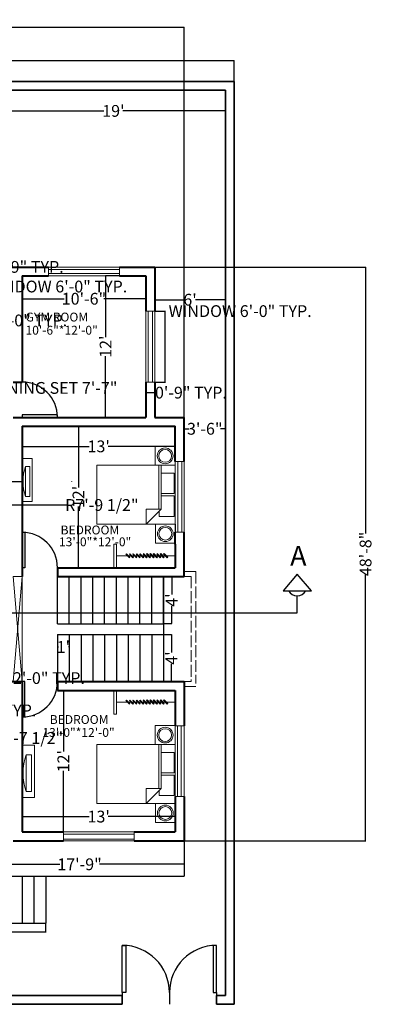
# Model space of a CAD drawing. Units: inches. Extents: x 1146 to 2917, y 889 to 2437.
# Tile 9 of 13: x 1792 to 2152, y 1432 to 2434. Entities that reach past the tile are written whole.
import ezdxf

# ---------------------------------------------------------------- set-up
doc = ezdxf.new("R2010")
doc.units = ezdxf.units.IN
doc.header["$MEASUREMENT"] = 0
doc.linetypes.add('ACAD_ISO02W100', pattern=[15, 12, -3])
for name, color, linetype, lineweight in [('A-ANNO-DIMS', 2, 'Continuous', 18), ('A-ANNO-SYMB', 7, 'Continuous', 25), ('A-AREA-IDEN', 7, 'Continuous', 18), ('A-FLOR-CASE', 9, 'Continuous', 20), ('A-FURN', 9, 'Continuous', 18), ('A-SITE-GATE', 10, 'Continuous', 25), ('A-SITE-WALL', 7, 'Continuous', 35), ('curtain wall', 70, 'ACAD_ISO02W100', 18), ('door', 10, 'Continuous', 25), ('openings', 130, 'Continuous', 18), ('staircase', 6, 'Continuous', 25), ('wall', 7, 'Continuous', 40), ('window', 5, 'Continuous', 18)]:
    doc.layers.add(name, color=color, linetype=linetype, lineweight=lineweight)
doc.styles.get("Standard").update_dxf_attribs({"font": 'arial.ttf'})
doc.dimstyles.new('Copy of Standard', dxfattribs={"dimtxt": 24, "dimasz": 0.18, "dimexe": 0.18, "dimexo": 0.0625, "dimgap": 0.09, "dimtad": 0, "dimtoh": 1, "dimdec": 1, "dimzin": 0, "dimdsep": 46, "dimlunit": 4, "dimtxsty": 'Standard', "dimcen": 0.09, "dimadec": 0, "dimazin": 0, "dimtfac": 1, "dimtdec": 1, "dimtofl": 0, "dimtmove": 0, "dimatfit": 3, "dimfxl": 1, "dimtolj": 1, "dimtzin": 0, "dimarcsym": 0})
doc.dimstyles.get("Standard").update_dxf_attribs({"dimtxt": 12, "dimasz": 0.18, "dimexe": 0.18, "dimexo": 0.0625, "dimgap": 0.09, "dimtad": 0, "dimtoh": 1, "dimdec": 1, "dimzin": 0, "dimdsep": 46, "dimlunit": 4, "dimtxsty": 'Standard', "dimcen": 0.09, "dimadec": 0, "dimazin": 0, "dimtfac": 1, "dimtdec": 1, "dimtofl": 0, "dimtmove": 0, "dimatfit": 3, "dimfxl": 1, "dimtolj": 1, "dimtzin": 0, "dimarcsym": 0})

# ---------------------------------------------------------------- blocks, each defined once
blk = doc.blocks.new('*D7')
at = {"layer": 'A-ANNO-DIMS', "color": 0, "lineweight": -2, "transparency": 16777216}
for p, q in [((1929.1, 2182.3), (1929.1, 2149)), ((2001.1, 2182.3), (2001.1, 2149)), ((1929.3, 2149.2), (1959.5, 2149.2)), ((2001, 2149.2), (1970.8, 2149.2))]:
    blk.add_line(p, q, dxfattribs=at)
at = {"layer": 'A-ANNO-DIMS', "color": 0, "transparency": 16777216}
for points in [[(1929.3, 2149.2), (1929.3, 2149.1), (1929.1, 2149.2)], [(2001, 2149.2), (2001, 2149.1), (2001.1, 2149.2)]]:
    blk.add_solid(points, dxfattribs=at)
at = {"layer": 'Defpoints', "color": 0, "transparency": 16777216}
for p in [(1929.1, 2182.4), (2001.1, 2182.4), (2001.1, 2149.2)]:
    blk.add_point(p, dxfattribs=at)
at = {"layer": 'A-ANNO-DIMS', "color": 0, "transparency": 16777216, "insert": (1965.1, 2149.2), "char_height": 12, "attachment_point": 5}
blk.add_mtext("\\A1;6'", dxfattribs=at)
blk = doc.blocks.new('*D8')
at = {"layer": 'A-ANNO-DIMS', "color": 0, "lineweight": -2, "transparency": 16777216}
for p, q in [((1794.1, 2020.3), (1794.1, 1999.8)), ((1950.1, 2020.3), (1950.1, 1999.8)), ((1794.3, 1999.9), (1862.4, 1999.9)), ((1950, 1999.9), (1881.8, 1999.9))]:
    blk.add_line(p, q, dxfattribs=at)
at = {"layer": 'A-ANNO-DIMS', "color": 0, "transparency": 16777216}
for points in [[(1794.3, 2000), (1794.3, 1999.9), (1794.1, 1999.9)], [(1950, 2000), (1950, 1999.9), (1950.1, 1999.9)]]:
    blk.add_solid(points, dxfattribs=at)
at = {"layer": 'Defpoints', "color": 0, "transparency": 16777216}
for p in [(1794.1, 2020.4), (1950.1, 2020.4), (1950.1, 1999.9)]:
    blk.add_point(p, dxfattribs=at)
at = {"layer": 'A-ANNO-DIMS', "color": 0, "transparency": 16777216, "insert": (1872.1, 1999.9), "char_height": 12, "attachment_point": 5}
blk.add_mtext("\\A1;13'", dxfattribs=at)
blk = doc.blocks.new('*D11')
at = {"layer": 'A-ANNO-DIMS', "color": 0, "lineweight": -2, "transparency": 16777216}
for p, q in [((1746.1, 1598.3), (1746.1, 1574.2)), ((1959.1, 1598.3), (1959.1, 1574.2)), ((1746.3, 1574.4), (1832.5, 1574.4)), ((1959, 1574.4), (1872.8, 1574.4))]:
    blk.add_line(p, q, dxfattribs=at)
at = {"layer": 'A-ANNO-DIMS', "color": 0, "transparency": 16777216}
for points in [[(1746.3, 1574.4), (1746.3, 1574.4), (1746.1, 1574.4)], [(1959, 1574.4), (1959, 1574.4), (1959.1, 1574.4)]]:
    blk.add_solid(points, dxfattribs=at)
at = {"layer": 'Defpoints', "color": 0, "transparency": 16777216}
for p in [(1746.1, 1598.4), (1959.1, 1598.4), (1959.1, 1574.4)]:
    blk.add_point(p, dxfattribs=at)
at = {"layer": 'A-ANNO-DIMS', "color": 0, "transparency": 16777216, "insert": (1852.6, 1574.4), "char_height": 12, "attachment_point": 5}
blk.add_mtext('\\A1;17\'-9"', dxfattribs=at)
blk = doc.blocks.new('*D14')
at = {"layer": 'A-ANNO-DIMS', "color": 0, "lineweight": -2, "transparency": 16777216}
for p, q in [((1602.1, 1514.3), (1602.1, 1505.1)), ((1818.1, 1514.3), (1818.1, 1505.1)), ((1602.3, 1505.3), (1700.4, 1505.3)), ((1818, 1505.3), (1719.8, 1505.3))]:
    blk.add_line(p, q, dxfattribs=at)
at = {"layer": 'A-ANNO-DIMS', "color": 0, "transparency": 16777216}
for points in [[(1602.3, 1505.3), (1602.3, 1505.2), (1602.1, 1505.3)], [(1818, 1505.3), (1818, 1505.2), (1818.1, 1505.3)]]:
    blk.add_solid(points, dxfattribs=at)
at = {"layer": 'Defpoints', "color": 0, "transparency": 16777216}
for p in [(1602.1, 1514.4), (1818.1, 1514.4), (1818.1, 1505.3)]:
    blk.add_point(p, dxfattribs=at)
at = {"layer": 'A-ANNO-DIMS', "color": 0, "transparency": 16777216, "insert": (1710.1, 1505.3), "char_height": 12, "attachment_point": 5}
blk.add_mtext("\\A1;18'", dxfattribs=at)
blk = doc.blocks.new('*U20')
for p, q in [((0, 0), (0, 6)), ((24, 0), (24, 6))]:
    blk.add_line(p, q)
blk.add_lwpolyline([(0, 0), (0, -24), (1.75, -24), (1.75, 0)], close=True)
blk.add_arc((0, 0), 24, 270, 0)
blk = doc.blocks.new('*U17')
for p, q in [((0, 0), (0, -6)), ((24, 0), (24, -6))]:
    blk.add_line(p, q)
blk.add_lwpolyline([(0, 0), (0, 24), (1.75, 24), (1.75, 0)], close=True)
blk.add_arc((0, 0), 24, 0, 90)
blk = doc.blocks.new('*U23')
for p, q in [((0, 0), (0, 6)), ((24, 0), (24, 6))]:
    blk.add_line(p, q)
blk.add_lwpolyline([(0, 0), (0, -24), (1.75, -24), (1.75, 0)], close=True)
blk.add_arc((0, 0), 24, 270, 0)
blk = doc.blocks.new('*U18')
for p, q in [((-24, 0), (-24, -6)), ((0, 0), (0, -6))]:
    blk.add_line(p, q)
blk.add_lwpolyline([(0, 0), (0, 24), (-1.75, 24), (-1.75, 0)], close=True)
blk.add_arc((0, 0), 24, 90, 180)
blk = doc.blocks.new('*D28')
at = {"layer": 'A-ANNO-DIMS', "color": 0, "lineweight": -2, "transparency": 16777216}
for p, q in [((1920.1, 2173.4), (1879, 2173.4)), ((1879.1, 2173.2), (1879.1, 2111.1)), ((1879.1, 2029.6), (1879.1, 2091.7)), ((1920.1, 2029.4), (1879, 2029.4))]:
    blk.add_line(p, q, dxfattribs=at)
at = {"layer": 'A-ANNO-DIMS', "color": 0, "transparency": 16777216}
for points in [[(1879.1, 2173.2), (1879.2, 2173.2), (1879.1, 2173.4)], [(1879.1, 2029.6), (1879.2, 2029.6), (1879.1, 2029.4)]]:
    blk.add_solid(points, dxfattribs=at)
at = {"layer": 'Defpoints', "color": 0, "transparency": 16777216}
for p in [(1920.1, 2173.4), (1879.1, 2029.4), (1920.1, 2029.4)]:
    blk.add_point(p, dxfattribs=at)
at = {"layer": 'A-ANNO-DIMS', "color": 0, "transparency": 16777216, "insert": (1879.1, 2101.4), "char_height": 12, "attachment_point": 5, "rotation": 90}
blk.add_mtext("\\A1;12'", dxfattribs=at)
blk = doc.blocks.new('*D29')
at = {"layer": 'A-ANNO-DIMS', "color": 0, "lineweight": -2, "transparency": 16777216}
for p, q in [((1794.1, 2173.3), (1794.1, 2150)), ((1920.1, 2173.3), (1920.1, 2150)), ((1794.3, 2150.2), (1837, 2150.2)), ((1920, 2150.2), (1877.3, 2150.2))]:
    blk.add_line(p, q, dxfattribs=at)
at = {"layer": 'A-ANNO-DIMS', "color": 0, "transparency": 16777216}
for points in [[(1794.3, 2150.2), (1794.3, 2150.2), (1794.1, 2150.2)], [(1920, 2150.2), (1920, 2150.2), (1920.1, 2150.2)]]:
    blk.add_solid(points, dxfattribs=at)
at = {"layer": 'Defpoints', "color": 0, "transparency": 16777216}
for p in [(1794.1, 2173.4), (1920.1, 2173.4), (1920.1, 2150.2)]:
    blk.add_point(p, dxfattribs=at)
at = {"layer": 'A-ANNO-DIMS', "color": 0, "transparency": 16777216, "insert": (1857.1, 2150.2), "char_height": 12, "attachment_point": 5}
blk.add_mtext('\\A1;10\'-6"', dxfattribs=at)
blk = doc.blocks.new('*D34')
at = {"layer": 'A-ANNO-DIMS', "color": 0, "lineweight": -2, "transparency": 16777216}
for p, q in [((1938.2, 1867.4), (1946.6, 1867.4)), ((1946.4, 1867.2), (1946.4, 1849.2)), ((1946.4, 1819.6), (1946.4, 1837.5)), ((1938.2, 1819.4), (1946.6, 1819.4))]:
    blk.add_line(p, q, dxfattribs=at)
at = {"layer": 'A-ANNO-DIMS', "color": 0, "transparency": 16777216}
for points in [[(1946.4, 1867.2), (1946.4, 1867.2), (1946.4, 1867.4)], [(1946.4, 1819.6), (1946.4, 1819.6), (1946.4, 1819.4)]]:
    blk.add_solid(points, dxfattribs=at)
at = {"layer": 'Defpoints', "color": 0, "transparency": 16777216}
for p in [(1938.1, 1867.4), (1938.1, 1819.4), (1946.4, 1819.4)]:
    blk.add_point(p, dxfattribs=at)
at = {"layer": 'A-ANNO-DIMS', "color": 0, "transparency": 16777216, "insert": (1946.4, 1843.4), "char_height": 12, "attachment_point": 5, "rotation": 90}
blk.add_mtext("\\A1;4'", dxfattribs=at)
blk = doc.blocks.new('*D35')
at = {"layer": 'A-ANNO-DIMS', "color": 0, "lineweight": -2, "transparency": 16777216}
for p, q in [((1938.2, 1808.4), (1946.3, 1808.4)), ((1946.1, 1808.2), (1946.1, 1790.2)), ((1946.1, 1760.6), (1946.1, 1778.5)), ((1938.2, 1760.4), (1946.3, 1760.4))]:
    blk.add_line(p, q, dxfattribs=at)
at = {"layer": 'A-ANNO-DIMS', "color": 0, "transparency": 16777216}
for points in [[(1946.1, 1808.2), (1946.2, 1808.2), (1946.1, 1808.4)], [(1946.1, 1760.6), (1946.2, 1760.6), (1946.1, 1760.4)]]:
    blk.add_solid(points, dxfattribs=at)
at = {"layer": 'Defpoints', "color": 0, "transparency": 16777216}
for p in [(1938.1, 1808.4), (1938.1, 1760.4), (1946.1, 1760.4)]:
    blk.add_point(p, dxfattribs=at)
at = {"layer": 'A-ANNO-DIMS', "color": 0, "transparency": 16777216, "insert": (1946.1, 1784.4), "char_height": 12, "attachment_point": 5, "rotation": 90}
blk.add_mtext("\\A1;4'", dxfattribs=at)
blk = doc.blocks.new('*D36')
at = {"layer": 'A-ANNO-DIMS', "color": 0, "lineweight": -2, "transparency": 16777216}
for p, q in [((1830.1, 1808.3), (1830.1, 1795.5)), ((1842.1, 1808.3), (1842.1, 1795.5)), ((1830.3, 1795.7), (1831.1, 1795.7)), ((1842, 1795.7), (1841.2, 1795.7))]:
    blk.add_line(p, q, dxfattribs=at)
at = {"layer": 'A-ANNO-DIMS', "color": 0, "transparency": 16777216}
for points in [[(1830.3, 1795.7), (1830.3, 1795.6), (1830.1, 1795.7)], [(1842, 1795.7), (1842, 1795.6), (1842.1, 1795.7)]]:
    blk.add_solid(points, dxfattribs=at)
at = {"layer": 'Defpoints', "color": 0, "transparency": 16777216}
for p in [(1830.1, 1808.4), (1842.1, 1808.4), (1842.1, 1795.7)]:
    blk.add_point(p, dxfattribs=at)
at = {"layer": 'A-ANNO-DIMS', "color": 0, "transparency": 16777216, "insert": (1836.1, 1795.7), "char_height": 12, "attachment_point": 5}
blk.add_mtext("\\A1;1'", dxfattribs=at)
blk = doc.blocks.new('*D37')
at = {"layer": 'A-ANNO-DIMS', "color": 0, "lineweight": -2, "transparency": 16777216}
for p, q in [((1959.1, 2029.3), (1959.1, 2017.6)), ((2001.1, 2029.3), (2001.1, 2017.6)), ((1959.3, 2017.8), (1964.1, 2017.8)), ((2001, 2017.8), (1996.2, 2017.8))]:
    blk.add_line(p, q, dxfattribs=at)
at = {"layer": 'A-ANNO-DIMS', "color": 0, "transparency": 16777216}
for points in [[(1959.3, 2017.8), (1959.3, 2017.8), (1959.1, 2017.8)], [(2001, 2017.8), (2001, 2017.8), (2001.1, 2017.8)]]:
    blk.add_solid(points, dxfattribs=at)
at = {"layer": 'Defpoints', "color": 0, "transparency": 16777216}
for p in [(1959.1, 2029.4), (2001.1, 2029.4), (2001.1, 2017.8)]:
    blk.add_point(p, dxfattribs=at)
at = {"layer": 'A-ANNO-DIMS', "color": 0, "transparency": 16777216, "insert": (1980.1, 2017.8), "char_height": 12, "attachment_point": 5}
blk.add_mtext('\\A1;3\'-6"', dxfattribs=at)
blk = doc.blocks.new('*D42')
at = {"layer": 'A-ANNO-DIMS', "color": 0, "lineweight": -2, "transparency": 16777216}
for p, q in [((1830.2, 1751.4), (1836.3, 1751.4)), ((1836.1, 1751.2), (1836.1, 1689.1)), ((1836.1, 1607.6), (1836.1, 1669.7)), ((1830.2, 1607.4), (1836.3, 1607.4))]:
    blk.add_line(p, q, dxfattribs=at)
at = {"layer": 'A-ANNO-DIMS', "color": 0, "transparency": 16777216}
for points in [[(1836.1, 1751.2), (1836.2, 1751.2), (1836.1, 1751.4)], [(1836.1, 1607.6), (1836.2, 1607.6), (1836.1, 1607.4)]]:
    blk.add_solid(points, dxfattribs=at)
at = {"layer": 'Defpoints', "color": 0, "transparency": 16777216}
for p in [(1830.1, 1751.4), (1830.1, 1607.4), (1836.1, 1607.4)]:
    blk.add_point(p, dxfattribs=at)
at = {"layer": 'A-ANNO-DIMS', "color": 0, "transparency": 16777216, "insert": (1836.1, 1679.4), "char_height": 12, "attachment_point": 5, "rotation": 90}
blk.add_mtext("\\A1;12'", dxfattribs=at)
blk = doc.blocks.new('*D43')
at = {"layer": 'A-ANNO-DIMS', "color": 0, "lineweight": -2, "transparency": 16777216}
for p, q in [((1794.1, 1607.5), (1794.1, 1623.1)), ((1794.3, 1623), (1862.4, 1623)), ((1950, 1623), (1881.8, 1623)), ((1950.1, 1607.5), (1950.1, 1623.1))]:
    blk.add_line(p, q, dxfattribs=at)
at = {"layer": 'A-ANNO-DIMS', "color": 0, "transparency": 16777216}
for points in [[(1794.3, 1623), (1794.3, 1622.9), (1794.1, 1623)], [(1950, 1623), (1950, 1622.9), (1950.1, 1623)]]:
    blk.add_solid(points, dxfattribs=at)
at = {"layer": 'Defpoints', "color": 0, "transparency": 16777216}
for p in [(1950.1, 1623), (1794.1, 1607.4), (1950.1, 1607.4)]:
    blk.add_point(p, dxfattribs=at)
at = {"layer": 'A-ANNO-DIMS', "color": 0, "transparency": 16777216, "insert": (1872.1, 1623), "char_height": 12, "attachment_point": 5}
blk.add_mtext("\\A1;13'", dxfattribs=at)
blk = doc.blocks.new('Bed - Queen')
for p, q in [((0, -80.00003), (0, 0)), ((0, 0), (59.99999, 0)), ((59.99999, 0), (59.99999, -80.00003)), ((7.99999, -1.2), (28.79998, -1.2)), ((7.99999, -14.4), (7.99999, -1.2)), ((28.79998, -1.2), (28.79998, -14.4)), ((31.19999, -1.2), (51.99999, -1.2)), ((31.19999, -14.4), (31.19999, -1.2)), ((51.99999, -1.2), (51.99999, -16.4)), ((0, -14.4), (44.8, -14.4)), ((44.8, -16.8), (0, -16.8)), ((59.99999, -29.6), (44.8, -14.4)), ((44.8, -14.4), (44.8, -29.6)), ((51.99999, -16.4), (46.79936, -16.4)), ((44.8, -29.6), (59.99999, -29.6)), ((59.99999, -80.00003), (0, -80.00003))]:
    blk.add_line(p, q)
blk = doc.blocks.new('*D48')
at = {"layer": 'A-ANNO-DIMS', "color": 0, "lineweight": -2, "transparency": 16777216}
for p, q in [((1950.1, 2020.4), (1851.3, 2020.4)), ((1851.5, 2020.2), (1851.5, 1958.1)), ((1851.5, 1876.6), (1851.5, 1938.7)), ((1950.1, 1876.4), (1851.3, 1876.4))]:
    blk.add_line(p, q, dxfattribs=at)
at = {"layer": 'A-ANNO-DIMS', "color": 0, "transparency": 16777216}
for points in [[(1851.5, 2020.2), (1851.6, 2020.2), (1851.5, 2020.4)], [(1851.5, 1876.6), (1851.6, 1876.6), (1851.5, 1876.4)]]:
    blk.add_solid(points, dxfattribs=at)
at = {"layer": 'Defpoints', "color": 0, "transparency": 16777216}
for p in [(1950.1, 2020.4), (1851.5, 1876.4), (1950.1, 1876.4)]:
    blk.add_point(p, dxfattribs=at)
at = {"layer": 'A-ANNO-DIMS', "color": 0, "transparency": 16777216, "insert": (1851.5, 1948.4), "char_height": 12, "attachment_point": 5, "rotation": 90}
blk.add_mtext("\\A1;12'", dxfattribs=at)
blk = doc.blocks.new('*D51')
at = {"layer": 'A-ANNO-DIMS', "color": 0, "lineweight": -2, "transparency": 16777216}
for p, q in [((1773.1, 2362.3), (1773.1, 2341.2)), ((2001.1, 2362.3), (2001.1, 2341.2)), ((1773.3, 2341.4), (1877.4, 2341.4)), ((2001, 2341.4), (1896.8, 2341.4))]:
    blk.add_line(p, q, dxfattribs=at)
at = {"layer": 'A-ANNO-DIMS', "color": 0, "transparency": 16777216}
for points in [[(1773.3, 2341.4), (1773.3, 2341.4), (1773.1, 2341.4)], [(2001, 2341.4), (2001, 2341.4), (2001.1, 2341.4)]]:
    blk.add_solid(points, dxfattribs=at)
at = {"layer": 'Defpoints', "color": 0, "transparency": 16777216}
for p in [(1773.1, 2362.4), (2001.1, 2362.4), (2001.1, 2341.4)]:
    blk.add_point(p, dxfattribs=at)
at = {"layer": 'A-ANNO-DIMS', "color": 0, "transparency": 16777216, "insert": (1887.1, 2341.4), "char_height": 12, "attachment_point": 5}
blk.add_mtext("\\A1;19'", dxfattribs=at)
blk = doc.blocks.new('*D53')
at = {"layer": 'A-ANNO-DIMS', "color": 0, "lineweight": -2, "transparency": 16777216}
for p, q in [((1305.1, 2371.5), (1305.1, 2392.7)), ((1305.3, 2392.5), (1616.3, 2392.5)), ((2010, 2392.5), (1698.9, 2392.5)), ((2010.1, 2371.5), (2010.1, 2392.7))]:
    blk.add_line(p, q, dxfattribs=at)
at = {"layer": 'A-ANNO-DIMS', "color": 0, "transparency": 16777216}
for points in [[(1305.3, 2392.5), (1305.3, 2392.5), (1305.1, 2392.5)], [(2010, 2392.5), (2010, 2392.5), (2010.1, 2392.5)]]:
    blk.add_solid(points, dxfattribs=at)
at = {"layer": 'Defpoints', "color": 0, "transparency": 16777216}
for p in [(2010.1, 2392.5), (1305.1, 2371.4), (2010.1, 2371.4)]:
    blk.add_point(p, dxfattribs=at)
at = {"layer": 'A-ANNO-DIMS', "color": 0, "transparency": 16777216, "insert": (1657.6, 2392.5), "char_height": 24, "attachment_point": 5}
blk.add_mtext('\\A1;58\'-9"', dxfattribs=at)
blk = doc.blocks.new('NIGHTSTAND-LAMP')
blk.add_lwpolyline([(0, 19.3), (20.4, 19.3), (20.4, 0), (0, 0)], close=True)
for radius in [8, 6.5]:
    blk.add_circle((10.2, 9.6), radius)
blk = doc.blocks.new('TV-CONSOLE')
for points in [[(0, 53.2), (12.5, 53.2), (12.5, 0), (0, 0)], [(3.1, 47.2), (8.5, 47.2), (8.5, 9.8), (3.1, 9.8)]]:
    blk.add_lwpolyline(points, close=True)
blk.add_arc((-49.2, 28.5), 60.7, 342.0216, 17.9784)
blk = doc.blocks.new('WINDOW-PLAN-72')
for points in [[(0, 72), (9, 72), (9, 0), (0, 0)], [(2.5, 0), (6.7, 0), (6.7, 72), (2.5, 72)]]:
    blk.add_lwpolyline(points, close=True)
blk = doc.blocks.new('WINDOW-PLAN-72-2')
for points in [[(0, 9), (72, 9), (72, 0), (0, 0)], [(0, 6.7), (72, 6.7), (72, 2.5), (0, 2.5)]]:
    blk.add_lwpolyline(points, close=True)
blk = doc.blocks.new('WINDOW-PLAN-72-3')
for points in [[(0, 72), (9, 72), (9, 0), (0, 0)], [(2.3, 72), (5.9, 72), (5.9, 0), (2.3, 0)]]:
    blk.add_lwpolyline(points, close=True)
blk = doc.blocks.new('WINDOW-PLAN-72-4')
for points in [[(0, 9), (72, 9), (72, 0), (0, 0)], [(0, 6.6), (72, 6.6), (72, 1.6), (0, 1.6)]]:
    blk.add_lwpolyline(points, close=True)
blk = doc.blocks.new('CLOSET-RAIL-HANGERS')
blk.add_line((2.4, 60), (2.4, 0))
for points in [[(0, 48.6), (3.6, 52.2), (4.2, 51.6), (0.6, 48)], [(0, 45.1), (3.6, 48.7), (4.2, 48.1), (0.6, 44.5)], [(0, 41.6), (3.6, 45.2), (4.2, 44.7), (0.6, 41.1)], [(0, 38.1), (3.6, 41.7), (4.2, 41.2), (0.6, 37.6)], [(0, 34.6), (3.6, 38.3), (4.2, 37.7), (0.6, 34.1)], [(0, 31.2), (3.6, 34.8), (4.2, 34.2), (0.6, 30.6)], [(0, 27.7), (3.7, 31.3), (4.2, 30.7), (0.6, 27.1)], [(0.1, 24.2), (3.7, 27.8), (4.2, 27.2), (0.6, 23.6)], [(0.1, 20.7), (3.7, 24.3), (4.2, 23.7), (0.6, 20.1)], [(0.1, 17.2), (3.7, 20.8), (4.2, 20.3), (0.6, 16.6)], [(0.1, 13.7), (3.7, 17.3), (4.3, 16.8), (0.6, 13.2)], [(0.1, 10.2), (3.7, 13.8), (4.3, 13.3), (0.7, 9.7)]]:
    blk.add_lwpolyline(points, close=True)
blk = doc.blocks.new('SECTION-HEAD')
for p, q in [((14.2, 39.3), (0, 22.6)), ((28.8, 22.6), (14.2, 39.3)), ((0, 22.6), (28.8, 22.6)), ((14.2, 0), (14.2, 17.2))]:
    blk.add_line(p, q)
blk.add_arc((14.2, 27), 9.77, 206.6471, 333.3529)
blk = doc.blocks.new('*D98')
at = {"layer": 'A-ANNO-DIMS', "color": 0, "lineweight": -2, "transparency": 16777216}
for p, q in [((1733.1, 1730.9), (1735.9, 1730.9)), ((1735.7, 1730.9), (1735.7, 1731.1)), ((1735.7, 1731.1), (1735.9, 1731.1)), ((1735.7, 1713.1), (1735.7, 1730.7)), ((1733.1, 1712.9), (1735.9, 1712.9))]:
    blk.add_line(p, q, dxfattribs=at)
at = {"layer": 'A-ANNO-DIMS', "color": 0, "transparency": 16777216}
for points in [[(1735.7, 1730.7), (1735.8, 1730.7), (1735.7, 1730.9)], [(1735.7, 1713.1), (1735.8, 1713.1), (1735.7, 1712.9)]]:
    blk.add_solid(points, dxfattribs=at)
at = {"layer": 'Defpoints', "color": 0, "transparency": 16777216}
for p in [(1733, 1730.9), (1735.7, 1730.9), (1733, 1712.9)]:
    blk.add_point(p, dxfattribs=at)
at = {"layer": 'A-ANNO-DIMS', "color": 0, "transparency": 16777216, "insert": (1772, 1731.1), "char_height": 12, "attachment_point": 5}
blk.add_mtext('\\A1;1\'-6" TYP.', dxfattribs=at)
blk = doc.blocks.new('*D103')
at = {"layer": 'A-ANNO-DIMS', "color": 0, "lineweight": -2, "transparency": 16777216}
for p, q in [((1929.2, 2137.4), (1940.1, 2137.4)), ((1939.9, 2137.4), (1939.9, 2137.6)), ((1939.9, 2137.6), (1940.1, 2137.6)), ((1939.9, 2065.6), (1939.9, 2137.2)), ((1929.2, 2065.4), (1940.1, 2065.4))]:
    blk.add_line(p, q, dxfattribs=at)
at = {"layer": 'A-ANNO-DIMS', "color": 0, "transparency": 16777216}
for points in [[(1939.9, 2137.2), (1940, 2137.2), (1939.9, 2137.4)], [(1939.9, 2065.6), (1940, 2065.6), (1939.9, 2065.4)]]:
    blk.add_solid(points, dxfattribs=at)
at = {"layer": 'Defpoints', "color": 0, "transparency": 16777216}
for p in [(1929.1, 2137.4), (1939.9, 2137.4), (1929.1, 2065.4)]:
    blk.add_point(p, dxfattribs=at)
at = {"layer": 'A-ANNO-DIMS', "color": 0, "transparency": 16777216, "insert": (2016.1, 2137.6), "char_height": 12, "attachment_point": 5}
blk.add_mtext('\\A1;WINDOW 6\'-0" TYP.', dxfattribs=at)
blk = doc.blocks.new('*D104')
at = {"layer": 'A-ANNO-DIMS', "color": 0, "lineweight": -2, "transparency": 16777216}
for p, q in [((1920.1, 2065.3), (1920.1, 2054.4)), ((1929.1, 2065.3), (1929.1, 2054.4)), ((1920.3, 2054.6), (1929, 2054.6)), ((1929.1, 2054.6), (1929.3, 2054.6))]:
    blk.add_line(p, q, dxfattribs=at)
at = {"layer": 'A-ANNO-DIMS', "color": 0, "transparency": 16777216}
for points in [[(1920.3, 2054.6), (1920.3, 2054.6), (1920.1, 2054.6)], [(1929, 2054.6), (1929, 2054.6), (1929.1, 2054.6)]]:
    blk.add_solid(points, dxfattribs=at)
at = {"layer": 'Defpoints', "color": 0, "transparency": 16777216}
for p in [(1920.1, 2065.4), (1929.1, 2065.4), (1929.1, 2054.6)]:
    blk.add_point(p, dxfattribs=at)
at = {"layer": 'A-ANNO-DIMS', "color": 0, "transparency": 16777216, "insert": (1966, 2054.6), "char_height": 12, "attachment_point": 5}
blk.add_mtext('\\A1;0\'-9" TYP.', dxfattribs=at)
blk = doc.blocks.new('*D105')
at = {"layer": 'A-ANNO-DIMS', "color": 0, "lineweight": -2, "transparency": 16777216}
for p, q in [((1649.8, 2127.9), (1659, 2127.9)), ((1658.8, 2127.9), (1658.8, 2128.1)), ((1658.8, 2128.1), (1659, 2128.1)), ((1658.8, 2068.1), (1658.8, 2127.7)), ((1649.8, 2067.9), (1659, 2067.9))]:
    blk.add_line(p, q, dxfattribs=at)
at = {"layer": 'A-ANNO-DIMS', "color": 0, "transparency": 16777216}
for points in [[(1658.7, 2127.7), (1658.8, 2127.7), (1658.8, 2127.9)], [(1658.7, 2068.1), (1658.8, 2068.1), (1658.8, 2067.9)]]:
    blk.add_solid(points, dxfattribs=at)
at = {"layer": 'Defpoints', "color": 0, "transparency": 16777216}
for p in [(1649.8, 2127.9), (1658.8, 2127.9), (1649.8, 2067.9)]:
    blk.add_point(p, dxfattribs=at)
at = {"layer": 'A-ANNO-DIMS', "color": 0, "transparency": 16777216, "insert": (1752.4, 2128.1), "char_height": 12, "attachment_point": 5}
blk.add_mtext('\\A1;CLOSET RAIL 5\'-0" TYP.', dxfattribs=at)
blk = doc.blocks.new('*D111')
at = {"layer": 'A-ANNO-DIMS', "color": 0, "lineweight": -2, "transparency": 16777216}
for p, q in [((1680.1, 2173.3), (1680.1, 2162.4)), ((1752.1, 2173.3), (1752.1, 2162.4)), ((1680.3, 2162.6), (1752, 2162.6)), ((1752.1, 2162.6), (1752.3, 2162.6))]:
    blk.add_line(p, q, dxfattribs=at)
at = {"layer": 'A-ANNO-DIMS', "color": 0, "transparency": 16777216}
for points in [[(1680.3, 2162.6), (1680.3, 2162.6), (1680.1, 2162.6)], [(1752, 2162.6), (1752, 2162.6), (1752.1, 2162.6)]]:
    blk.add_solid(points, dxfattribs=at)
at = {"layer": 'Defpoints', "color": 0, "transparency": 16777216}
for p in [(1680.1, 2173.4), (1752.1, 2173.4), (1752.1, 2162.6)]:
    blk.add_point(p, dxfattribs=at)
at = {"layer": 'A-ANNO-DIMS', "color": 0, "transparency": 16777216, "insert": (1828.3, 2162.6), "char_height": 12, "attachment_point": 5}
blk.add_mtext('\\A1;WINDOW 6\'-0" TYP.', dxfattribs=at)
blk = doc.blocks.new('*D112')
at = {"layer": 'A-ANNO-DIMS', "color": 0, "lineweight": -2, "transparency": 16777216}
for p, q in [((1752.2, 2182.4), (1763.1, 2182.4)), ((1762.9, 2182.4), (1762.9, 2182.6)), ((1762.9, 2182.6), (1763.1, 2182.6)), ((1762.9, 2173.6), (1762.9, 2182.2)), ((1752.2, 2173.4), (1763.1, 2173.4))]:
    blk.add_line(p, q, dxfattribs=at)
at = {"layer": 'A-ANNO-DIMS', "color": 0, "transparency": 16777216}
for points in [[(1762.9, 2182.2), (1763, 2182.2), (1762.9, 2182.4)], [(1762.9, 2173.6), (1763, 2173.6), (1762.9, 2173.4)]]:
    blk.add_solid(points, dxfattribs=at)
at = {"layer": 'Defpoints', "color": 0, "transparency": 16777216}
for p in [(1752.1, 2182.4), (1762.9, 2182.4), (1752.1, 2173.4)]:
    blk.add_point(p, dxfattribs=at)
at = {"layer": 'A-ANNO-DIMS', "color": 0, "transparency": 16777216, "insert": (1799.8, 2182.6), "char_height": 12, "attachment_point": 5}
blk.add_mtext('\\A1;0\'-9" TYP.', dxfattribs=at)
blk = doc.blocks.new('*D117')
at = {"layer": 'A-ANNO-DIMS', "color": 0, "lineweight": -2, "transparency": 16777216}
for p, q in [((1671.1, 1760.5), (1671.1, 1764.2)), ((1671.3, 1764), (1695, 1764)), ((1695.1, 1760.5), (1695.1, 1764.2)), ((1695.1, 1764), (1695.3, 1764))]:
    blk.add_line(p, q, dxfattribs=at)
at = {"layer": 'A-ANNO-DIMS', "color": 0, "transparency": 16777216}
for points in [[(1671.3, 1764), (1671.3, 1764), (1671.1, 1764)], [(1695, 1764), (1695, 1764), (1695.1, 1764)]]:
    blk.add_solid(points, dxfattribs=at)
at = {"layer": 'Defpoints', "color": 0, "transparency": 16777216}
for p in [(1671.1, 1760.4), (1695.1, 1764), (1695.1, 1760.4)]:
    blk.add_point(p, dxfattribs=at)
at = {"layer": 'A-ANNO-DIMS', "color": 0, "transparency": 16777216, "insert": (1778.5, 1764), "char_height": 12, "attachment_point": 5}
blk.add_mtext('\\A1;SIDELIGHT 2\'-0" TYP.', dxfattribs=at)
blk = doc.blocks.new('*D119')
at = {"layer": 'A-ANNO-DIMS', "color": 0, "lineweight": -2, "transparency": 16777216}
for p, q in [((1669.7, 2073), (1669.7, 2059.2)), ((1760.7, 2073), (1760.7, 2059.2)), ((1669.9, 2059.4), (1760.5, 2059.4)), ((1760.7, 2059.4), (1760.9, 2059.4))]:
    blk.add_line(p, q, dxfattribs=at)
at = {"layer": 'A-ANNO-DIMS', "color": 0, "transparency": 16777216}
for points in [[(1669.9, 2059.4), (1669.9, 2059.4), (1669.7, 2059.4)], [(1760.5, 2059.4), (1760.5, 2059.4), (1760.7, 2059.4)]]:
    blk.add_solid(points, dxfattribs=at)
at = {"layer": 'Defpoints', "color": 0, "transparency": 16777216}
for p in [(1669.7, 2073.1), (1760.7, 2073.1), (1760.7, 2059.4)]:
    blk.add_point(p, dxfattribs=at)
at = {"layer": 'A-ANNO-DIMS', "color": 0, "transparency": 16777216, "insert": (1826.9, 2059.4), "char_height": 12, "attachment_point": 5}
blk.add_mtext('\\A1;DINING SET 7\'-7"', dxfattribs=at)
blk = doc.blocks.new('*D168')
at = {"layer": 'A-ANNO-DIMS', "color": 0, "lineweight": -2, "transparency": 16777216}
for p, q in [((1431.1, 2029.5), (1431.1, 2426.6)), ((1431.3, 2426.4), (1674.2, 2426.4)), ((1959, 2426.4), (1716.1, 2426.4)), ((1959.1, 2029.5), (1959.1, 2426.6))]:
    blk.add_line(p, q, dxfattribs=at)
at = {"layer": 'A-ANNO-DIMS', "color": 0, "transparency": 16777216}
for points in [[(1431.3, 2426.4), (1431.3, 2426.4), (1431.1, 2426.4)], [(1959, 2426.4), (1959, 2426.4), (1959.1, 2426.4)]]:
    blk.add_solid(points, dxfattribs=at)
at = {"layer": 'Defpoints', "color": 0, "transparency": 16777216}
for p in [(1959.1, 2426.4), (1431.1, 2029.4), (1959.1, 2029.4)]:
    blk.add_point(p, dxfattribs=at)
at = {"layer": 'A-ANNO-DIMS', "color": 0, "transparency": 16777216, "insert": (1695.1, 2426.4), "char_height": 12, "attachment_point": 5}
blk.add_mtext('\\A1;44\'-0"', dxfattribs=at)
blk = doc.blocks.new('*D169')
at = {"layer": 'A-ANNO-DIMS', "color": 0, "lineweight": -2, "transparency": 16777216}
for p, q in [((1929.2, 2182.4), (2144, 2182.4)), ((2143.8, 2182.2), (2143.8, 1911.3)), ((2143.8, 1598.6), (2143.8, 1869.4)), ((1959.2, 1598.4), (2144, 1598.4))]:
    blk.add_line(p, q, dxfattribs=at)
at = {"layer": 'A-ANNO-DIMS', "color": 0, "transparency": 16777216}
for points in [[(2143.8, 2182.2), (2143.9, 2182.2), (2143.8, 2182.4)], [(2143.8, 1598.6), (2143.9, 1598.6), (2143.8, 1598.4)]]:
    blk.add_solid(points, dxfattribs=at)
at = {"layer": 'Defpoints', "color": 0, "transparency": 16777216}
for p in [(1929.1, 2182.4), (2143.8, 2182.4), (1959.1, 1598.4)]:
    blk.add_point(p, dxfattribs=at)
at = {"layer": 'A-ANNO-DIMS', "color": 0, "transparency": 16777216, "insert": (2143.8, 1890.4), "char_height": 12, "attachment_point": 5, "rotation": 90}
blk.add_mtext('\\A1;48\'-8"', dxfattribs=at)
blk = doc.blocks.new('*D175')
at = {"layer": 'A-ANNO-DIMS', "color": 0, "lineweight": -2, "transparency": 16777216}
for p, q in [((1689.7, 1940.2), (1689.9, 1940.2)), ((1689.8, 1940.1), (1689.8, 1940.3)), ((1839.6, 1940.2), (1783.6, 1940.2))]:
    blk.add_line(p, q, dxfattribs=at)
at = {"layer": 'A-ANNO-DIMS', "color": 0, "transparency": 16777216}
blk.add_solid([(1783.6, 1940.2), (1783.6, 1940.2), (1783.4, 1940.2)], dxfattribs=at)
at = {"layer": 'Defpoints', "color": 0, "transparency": 16777216}
for p in [(1689.8, 1940.2), (1783.4, 1940.2)]:
    blk.add_point(p, dxfattribs=at)
at = {"layer": 'A-ANNO-DIMS', "color": 0, "transparency": 16777216, "insert": (1875.3, 1940.2), "char_height": 12, "attachment_point": 5}
blk.add_mtext('\\A1;R7\'-9 1/2"', dxfattribs=at)
blk = doc.blocks.new('*D177')
at = {"layer": 'A-ANNO-DIMS', "color": 0, "lineweight": -2, "transparency": 16777216}
for p, q in [((1765.2, 1964.2), (1794.9, 1964.2)), ((1844.8, 1964.1), (1844.8, 1964.3)), ((1844.8, 1964.2), (1844.9, 1964.2))]:
    blk.add_line(p, q, dxfattribs=at)
at = {"layer": 'A-ANNO-DIMS', "color": 0, "transparency": 16777216}
blk.add_solid([(1794.9, 1964.2), (1794.9, 1964.1), (1795.1, 1964.2)], dxfattribs=at)
at = {"layer": 'Defpoints', "color": 0, "transparency": 16777216}
for p in [(1795.1, 1964.2), (1844.8, 1964.2)]:
    blk.add_point(p, dxfattribs=at)
at = {"layer": 'A-ANNO-DIMS', "color": 0, "transparency": 16777216, "insert": (1743.4, 1964.2), "char_height": 12, "attachment_point": 5}
blk.add_mtext('\\A1;R4\'-2"', dxfattribs=at)
blk = doc.blocks.new('*D181')
at = {"layer": 'A-ANNO-DIMS', "color": 0, "lineweight": -2, "transparency": 16777216}
for p, q in [((1743.3, 1703), (1743.5, 1703)), ((1743.4, 1702.9), (1743.4, 1703.1)), ((1759, 1703), (1753.3, 1703))]:
    blk.add_line(p, q, dxfattribs=at)
at = {"layer": 'A-ANNO-DIMS', "color": 0, "transparency": 16777216}
blk.add_solid([(1753.3, 1703), (1753.3, 1703), (1753.1, 1703)], dxfattribs=at)
at = {"layer": 'Defpoints', "color": 0, "transparency": 16777216}
for p in [(1733.7, 1703), (1753.1, 1703)]:
    blk.add_point(p, dxfattribs=at)
at = {"layer": 'A-ANNO-DIMS', "color": 0, "transparency": 16777216, "insert": (1795.5, 1703), "char_height": 12, "attachment_point": 5}
blk.add_mtext('\\A1;∅1\'-7 1/2"', dxfattribs=at)

msp = doc.modelspace()

# ---------------------------------------------------------------- linework, layer by layer
at = {"layer": 'A-ANNO-SYMB'}
msp.add_line((1232.84, 1830.35), (2074.15, 1830.35), dxfattribs=at)
at = {"layer": 'A-FLOR-CASE'}
for p, q in [((1887.63, 1900.39), (1890.13, 1900.39)), ((1887.63, 1900.39), (1887.63, 1876.39)), ((1890.13, 1900.39), (1890.13, 1876.39)), ((1887.63, 1751.39), (1887.63, 1727.39)), ((1890.13, 1751.39), (1890.13, 1727.39)), ((1887.63, 1727.39), (1890.13, 1727.39))]:
    msp.add_line(p, q, dxfattribs=at)
at = {"layer": 'A-FURN'}
for points in [[(1804.43, 1943.89), (1794.13, 1943.89), (1794.13, 1987.55), (1804.43, 1987.55)], [(1801.86, 1948.81), (1797.48, 1948.81), (1797.48, 1979.54), (1801.86, 1979.54)]]:
    msp.add_lwpolyline(points, close=True, dxfattribs=at)
msp.add_arc((1844.84, 1964.17), 49.79, 162.0216, 197.9784, dxfattribs=at)
at = {"layer": 'A-SITE-WALL'}
for p, q in [((1305.13, 2371.39), (2010.13, 2371.39)), ((2010.13, 2371.39), (2010.13, 1431.89)), ((1773.13, 2362.39), (2001.13, 2362.39)), ((2001.13, 2362.39), (2001.13, 1440.89)), ((1464.13, 1440.89), (1896.13, 1440.89)), ((1896.13, 1440.89), (1896.13, 1431.89)), ((1992.13, 1440.89), (1992.13, 1431.89)), ((1992.13, 1440.89), (2001.13, 1440.89)), ((1464.13, 1431.89), (1896.13, 1431.89)), ((1992.13, 1431.89), (2010.13, 1431.89))]:
    msp.add_line(p, q, dxfattribs=at)
at = {"layer": 'curtain wall'}
for p, q in [((1959.13, 1872.39), (1971.13, 1872.39)), ((1959.13, 1867.39), (1966.13, 1867.39)), ((1966.13, 1867.39), (1966.13, 1760.39)), ((1971.13, 1872.39), (1971.13, 1762.39)), ((1966.13, 1760.39), (1959.13, 1760.39)), ((1971.13, 1755.39), (1959.13, 1755.39)), ((1971.13, 1758.39), (1971.13, 1762.39))]:
    msp.add_line(p, q, dxfattribs=at)
at = {"layer": 'openings'}
for p, q in [((1785.13, 1867.39), (1794.13, 1760.39)), ((1785.13, 1760.39), (1794.13, 1867.39)), ((1785.13, 1867.39), (1794.13, 1867.39)), ((1794.13, 1760.39), (1794.13, 1867.39)), ((1794.13, 1760.39), (1785.13, 1760.39))]:
    msp.add_line(p, q, dxfattribs=at)
at = {"layer": 'staircase'}
for p, q in [((1830.13, 1819.39), (1830.13, 1867.39)), ((1842.13, 1819.39), (1842.13, 1867.39)), ((1854.13, 1819.39), (1854.13, 1867.39)), ((1866.13, 1819.39), (1866.13, 1867.39)), ((1878.13, 1819.39), (1878.13, 1867.39)), ((1890.13, 1819.39), (1890.13, 1867.39)), ((1902.13, 1819.39), (1902.13, 1867.39)), ((1902.13, 1819.39), (1902.13, 1867.39)), ((1914.13, 1819.39), (1914.13, 1867.39)), ((1926.13, 1819.39), (1926.13, 1867.39)), ((1938.13, 1819.39), (1938.13, 1867.39)), ((1938.13, 1867.39), (1938.13, 1760.39)), ((1830.13, 1819.39), (1938.13, 1819.39)), ((1830.13, 1808.39), (1830.13, 1760.39)), ((1830.13, 1808.39), (1938.13, 1808.39)), ((1842.13, 1808.39), (1842.13, 1760.39)), ((1854.13, 1808.39), (1854.13, 1760.39)), ((1866.13, 1808.39), (1866.13, 1760.39)), ((1878.13, 1808.39), (1878.13, 1760.39)), ((1890.13, 1808.39), (1890.13, 1760.39)), ((1902.13, 1808.39), (1902.13, 1760.39)), ((1914.13, 1808.39), (1914.13, 1760.39)), ((1926.13, 1808.39), (1926.13, 1760.39)), ((1959.13, 1598.39), (1959.13, 1562.39)), ((1746.13, 1562.39), (1959.13, 1562.39)), ((1794.13, 1562.39), (1794.13, 1514.39)), ((1806.13, 1562.39), (1806.13, 1514.39)), ((1818.13, 1562.39), (1818.13, 1514.39)), ((1746.13, 1514.39), (1818.13, 1514.39))]:
    msp.add_line(p, q, dxfattribs=at)
at = {"layer": 'wall'}
for p, q in [((1752.13, 2182.39), (1821.13, 2182.39)), ((1893.13, 2182.39), (1929.13, 2182.39)), ((1929.13, 2182.39), (1929.13, 2137.39)), ((1794.13, 2173.39), (1794.13, 2065.39)), ((1794.13, 2173.39), (1821.13, 2173.39)), ((1893.13, 2173.39), (1920.13, 2173.39)), ((1920.13, 2173.39), (1920.13, 2137.39)), ((1785.13, 2065.39), (1794.13, 2065.39)), ((1920.13, 2065.39), (1920.13, 2029.39)), ((1929.13, 2065.39), (1929.13, 2029.39)), ((1785.13, 2029.39), (1920.13, 2029.39)), ((1929.13, 2029.39), (1959.13, 2029.39)), ((1959.13, 1984.39), (1959.13, 2029.39)), ((1794.13, 2020.39), (1794.13, 1867.39)), ((1794.13, 2020.39), (1929.13, 2020.39)), ((1929.13, 2020.39), (1950.13, 2020.39)), ((1950.13, 1984.39), (1950.13, 2020.39)), ((1950.13, 1900.39), (1950.13, 1912.39)), ((1959.13, 1867.39), (1959.13, 1912.39)), ((1950.13, 1900.39), (1950.13, 1876.39)), ((1830.13, 1876.39), (1830.13, 1867.39)), ((1830.13, 1876.39), (1950.13, 1876.39)), ((1830.13, 1867.39), (1950.13, 1867.39)), ((1950.13, 1867.39), (1959.13, 1867.39)), ((1737.13, 1760.39), (1794.13, 1760.39)), ((1794.13, 1760.39), (1794.13, 1607.39)), ((1830.13, 1760.39), (1830.13, 1751.39)), ((1830.13, 1760.39), (1950.13, 1760.39)), ((1950.13, 1760.39), (1959.13, 1760.39)), ((1959.13, 1760.39), (1959.13, 1715.39)), ((1830.13, 1751.39), (1950.13, 1751.39)), ((1950.13, 1751.39), (1950.13, 1715.39)), ((1950.13, 1643.39), (1950.13, 1607.39)), ((1959.13, 1643.39), (1959.13, 1598.39)), ((1794.13, 1607.39), (1836.13, 1607.39)), ((1908.13, 1607.39), (1950.13, 1607.39)), ((1785.13, 1598.39), (1836.13, 1598.39)), ((1908.13, 1598.39), (1959.13, 1598.39))]:
    msp.add_line(p, q, dxfattribs=at)

# ---------------------------------------------------------------- block references
at = {"layer": 'A-ANNO-SYMB'}
msp.add_blockref('SECTION-HEAD', (2060, 1830.35), dxfattribs=at)
at = {"layer": 'A-FLOR-CASE', "rotation": 269.9999999999962}
for p in [(1890.13, 1890.76), (1890.13, 1741.76)]:
    msp.add_blockref('CLOSET-RAIL-HANGERS', p, dxfattribs=at)
at = {"layer": 'A-FURN'}
for p in [(1929.59, 1980.64), (1929.77, 1901.36), (1929.59, 1696.32), (1929.77, 1617.05)]:
    msp.add_blockref('NIGHTSTAND-LAMP', p, dxfattribs=at)
for name, p, rotation in [('Bed - Queen', (1950.13, 1980.64), 270), ('TV-CONSOLE', (1806.68, 1695.68), 180), ('Bed - Queen', (1950.13, 1696.32), 270)]:
    msp.add_blockref(name, p, dxfattribs=dict(at, rotation=rotation))
at = {"layer": 'A-SITE-GATE', "xscale": 2, "yscale": 2, "zscale": 2}
for name, p in [('*U17', (1896.13, 1443.89)), ('*U18', (1992.13, 1443.89))]:
    msp.add_blockref(name, p, dxfattribs=at)
at = {"layer": 'door', "xscale": 1.499999999999961, "yscale": 1.499999999999961, "zscale": 1.499999999999961, "rotation": 90}
msp.add_blockref('*U20', (1794.13, 2029.39), dxfattribs=at)
at = {"layer": 'door', "xscale": 1.500000000000009, "yscale": 1.500000000000009, "zscale": 1.500000000000009}
for name, p in [('*U17', (1794.13, 1876.39)), ('*U23', (1794.13, 1760.39))]:
    msp.add_blockref(name, p, dxfattribs=at)
at = {"layer": 'window'}
for name, p in [('WINDOW-PLAN-72-2', (1821.13, 2173.39)), ('WINDOW-PLAN-72', (1920.13, 2065.39)), ('WINDOW-PLAN-72', (1950.13, 1912.39)), ('WINDOW-PLAN-72-3', (1950.13, 1643.39)), ('WINDOW-PLAN-72-4', (1836.13, 1598.39))]:
    msp.add_blockref(name, p, dxfattribs=at)

# ---------------------------------------------------------------- texts
at = {"layer": 'A-ANNO-SYMB', "insert": (2067.09, 1898.56), "char_height": 20, "attachment_point": 1}
msp.add_mtext_dynamic_manual_height_columns('A', width=22.084, gutter_width=1, heights=[0], dxfattribs=at)
at = {"layer": 'A-AREA-IDEN', "char_height": 9, "attachment_point": 1}
for s, width, insert in [('GYM ROOM', 74.6171, (1797.67, 2136.04)), ('10\'-6"*12\'-0"', 73.6169, (1797.58, 2122.65)), ('BEDROOM', 41.1689, (1833.32, 1919.28)), ('13\'-0"*12\'-0"', 70.5587, (1831.67, 1907.21)), ('BEDROOM', 41.1689, (1822.28, 1726.33)), ('13\'-0"*12\'-0"', 80.3479, (1814.77, 1713.14))]:
    msp.add_mtext_dynamic_manual_height_columns(s, width=width, gutter_width=1, heights=[0], dxfattribs=dict(at, insert=insert))

# ---------------------------------------------------------------- dimensions: what is measured, and where the dimension line sits
at = {"layer": 'A-ANNO-DIMS'}
dim = msp.add_linear_dim(base=(1959.13, 2426.39), p1=(1431.13, 2029.39), p2=(1959.13, 2029.39), dimstyle='Standard', override={"dimdec": 1, "dimlfac": 1, "dimrnd": 0, "dimzin": 1, "dimdsep": 46, "dimlunit": 4, "dimfrac": 2}, dxfattribs=at)
dim.commit()
dim.dimension.update_dxf_attribs({"geometry": '*D168', "text_midpoint": (1695.13, 2426.39)})
for p1, p2, distance, dimstyle, picture, middle in [((1305.13, 2371.39), (2010.13, 2371.39), 21.1, 'Copy of Standard', '*D53', (1657.63, 2392.49)), ((1773.13, 2362.39), (2001.13, 2362.39), -20.97, 'Standard', '*D51', (1887.13, 2341.42)), ((1929.13, 2182.39), (2001.13, 2182.39), -33.21, 'Standard', '*D7', (1965.13, 2149.18)), ((1794.13, 2173.39), (1920.13, 2173.39), -23.21, 'Standard', '*D29', (1857.13, 2150.18)), ((1920.13, 2173.39), (1920.13, 2029.39), -41, 'Standard', '*D28', (1879.13, 2101.39)), ((1959.13, 2029.39), (2001.13, 2029.39), -11.58, 'Standard', '*D37', (1980.13, 2017.81)), ((1950.13, 2020.39), (1950.13, 1876.39), -98.61, 'Standard', '*D48', (1851.53, 1948.39)), ((1938.13, 1867.39), (1938.13, 1819.39), 8.27, 'Standard', '*D34', (1946.4, 1843.39)), ((1830.13, 1808.39), (1842.13, 1808.39), -12.73, 'Standard', '*D36', (1836.13, 1795.66)), ((1938.13, 1808.39), (1938.13, 1760.39), 7.99, 'Standard', '*D35', (1946.12, 1784.39)), ((1830.13, 1751.39), (1830.13, 1607.39), 6, 'Standard', '*D42', (1836.13, 1679.39)), ((1794.13, 1607.39), (1950.13, 1607.39), 15.57, 'Standard', '*D43', (1872.13, 1622.96)), ((1746.13, 1598.39), (1959.13, 1598.39), -24, 'Standard', '*D11', (1852.63, 1574.39)), ((1602.13, 1514.39), (1818.13, 1514.39), -9.13, 'Standard', '*D14', (1710.13, 1505.26))]:
    dim = msp.add_aligned_dim(p1=p1, p2=p2, distance=distance, dimstyle=dimstyle, override={"dimclrd": 0, "dimclre": 0, "dimclrt": 0}, dxfattribs=at)
    dim.commit()
    dim.dimension.update_dxf_attribs({"geometry": picture, "text_midpoint": middle})
for base, p1, p2, text, picture, middle in [((1762.93, 2182.39), (1752.13, 2173.39), (1752.13, 2182.39), '<> TYP.', '*D112', (1799.78, 2182.57)), ((1658.77, 2127.89), (1649.77, 2067.89), (1649.77, 2127.89), 'CLOSET RAIL <> TYP.', '*D105', (1752.38, 2128.07)), ((1939.93, 2137.39), (1929.13, 2065.39), (1929.13, 2137.39), 'WINDOW <> TYP.', '*D103', (2016.13, 2137.57)), ((1735.72, 1730.9), (1733.03, 1712.94), (1733.03, 1730.9), '<> TYP.', '*D98', (1772, 1731.08))]:
    dim = msp.add_linear_dim(base=base, p1=p1, p2=p2, angle=90, text=text, dimstyle='Standard', override={"dimdec": 1, "dimlfac": 1, "dimrnd": 0, "dimzin": 1, "dimdsep": 46, "dimlunit": 4, "dimfrac": 2}, dxfattribs=at)
    dim.commit()
    dim.dimension.update_dxf_attribs({"geometry": picture, "text_midpoint": middle})
for base, p1, p2, text, picture, middle in [((1752.13, 2162.59), (1680.13, 2173.39), (1752.13, 2173.39), 'WINDOW <> TYP.', '*D111', (1828.33, 2162.59)), ((1760.67, 2059.42), (1669.67, 2073.07), (1760.67, 2073.07), 'DINING SET <>', '*D119', (1826.89, 2059.42)), ((1929.13, 2054.59), (1920.13, 2065.39), (1929.13, 2065.39), '<> TYP.', '*D104', (1965.98, 2054.59)), ((1695.13, 1763.99), (1671.13, 1760.39), (1695.13, 1760.39), 'SIDELIGHT <> TYP.', '*D117', (1778.52, 1763.99))]:
    dim = msp.add_linear_dim(base=base, p1=p1, p2=p2, text=text, dimstyle='Standard', override={"dimdec": 1, "dimlfac": 1, "dimrnd": 0, "dimzin": 1, "dimdsep": 46, "dimlunit": 4, "dimfrac": 2}, dxfattribs=at)
    dim.commit()
    dim.dimension.update_dxf_attribs({"geometry": picture, "text_midpoint": middle})
dim = msp.add_linear_dim(base=(2143.83, 2182.39), p1=(1959.13, 1598.39), p2=(1929.13, 2182.39), angle=90, dimstyle='Standard', override={"dimdec": 1, "dimlfac": 1, "dimrnd": 0, "dimzin": 1, "dimdsep": 46, "dimlunit": 4, "dimfrac": 2}, dxfattribs=at)
dim.commit()
dim.dimension.update_dxf_attribs({"geometry": '*D169', "text_midpoint": (2143.83, 1890.39)})
dim = msp.add_linear_dim(base=(1950.13, 1999.94), p1=(1794.13, 2020.39), p2=(1950.13, 2020.39), angle=0, dimstyle='Standard', override={"dimclrd": 0, "dimclre": 0, "dimclrt": 0}, dxfattribs=at)
dim.commit()
dim.dimension.update_dxf_attribs({"geometry": '*D8', "text_midpoint": (1872.13, 1999.94), "dimtype": 161})
for center, mpoint, picture, middle in [((1844.84, 1964.17), (1795.05, 1964.17), '*D177', (1765.18, 1964.17)), ((1689.83, 1940.2), (1783.41, 1940.2), '*D175', (1839.56, 1940.2))]:
    dim = msp.add_radius_dim(center=center, mpoint=mpoint, dimstyle='Standard', override={"dimdec": 1, "dimlfac": 1, "dimrnd": 0, "dimzin": 1, "dimdsep": 46, "dimlunit": 4, "dimfrac": 2}, dxfattribs=at)
    dim.commit()
    dim.dimension.update_dxf_attribs({"geometry": picture, "text_midpoint": middle, "dimtype": 164})
dim = msp.add_diameter_dim_2p(p1=(1733.6758, 1702.9975), p2=(1753.135, 1702.998), dimstyle='Standard', override={"dimdec": 1, "dimlfac": 1, "dimrnd": 0, "dimzin": 1, "dimdsep": 46, "dimlunit": 4, "dimfrac": 2}, dxfattribs=at)
dim.commit()
dim.dimension.update_dxf_attribs({"geometry": '*D181', "text_midpoint": (1758.9728, 1702.9981), "dimtype": 163})

doc.saveas('drawing.dxf')
